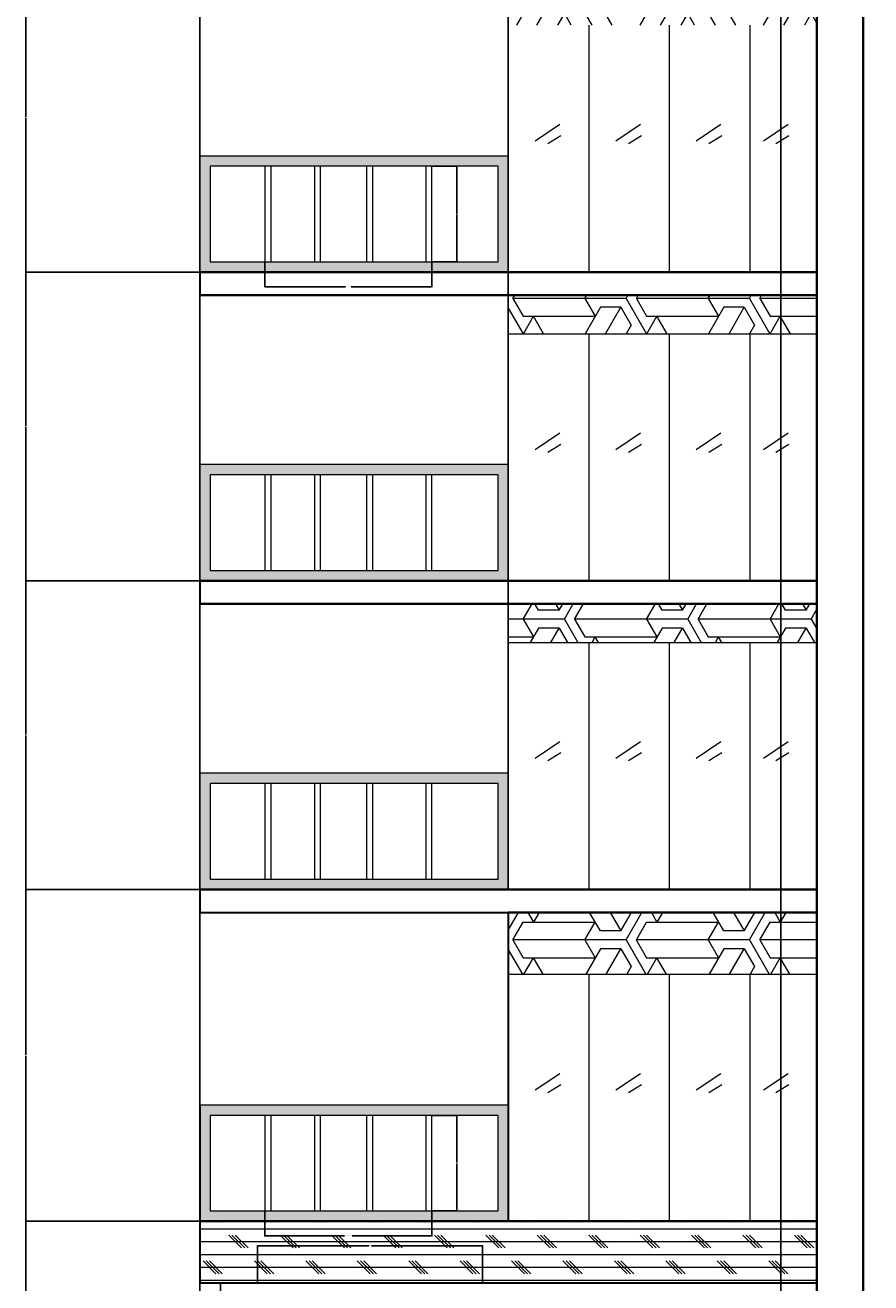
# Model space of a CAD drawing. Units: inches. Extents: x -38 to 698, y -57 to 1364.
# Tile 2 of 5: x -38 to 291, y 227 to 716. Entities that reach past the tile are written whole.
import ezdxf

# ---------------------------------------------------------------- set-up
doc = ezdxf.new("R2010")
doc.units = ezdxf.units.IN
doc.header["$MEASUREMENT"] = 0
for name, color, linetype, lineweight in [('A-ANNO-DIMS', 2, 'Continuous', 18), ('A-ELEV-PATT', 8, 'Continuous', 13), ('A-FLOR', 7, 'Continuous', 30), ('A-FLOR-HRAL', 7, 'Continuous', 20), ('A-GLAZ', 4, 'Continuous', 18), ('A-WALL', 7, 'Continuous', 35), ('A-WALL-PATT', 8, 'Continuous', 13)]:
    doc.layers.add(name, color=color, linetype=linetype, lineweight=lineweight)
doc.styles.get("Standard").update_dxf_attribs({"font": 'arial.ttf'})
doc.dimstyles.get("Standard").update_dxf_attribs({"dimtxt": 0.18, "dimasz": 0.18, "dimexe": 0.18, "dimexo": 0.0625, "dimgap": 0.09, "dimtad": 0, "dimtih": 1, "dimtoh": 1, "dimdec": 4, "dimzin": 0, "dimdsep": 46, "dimtxsty": 'Standard', "dimcen": 0.09, "dimadec": 0, "dimazin": 0, "dimtfac": 1, "dimtdec": 4, "dimtofl": 0, "dimtmove": 0, "dimatfit": 3, "dimfxl": 1, "dimtolj": 1, "dimtzin": 0, "dimarcsym": 0})

# ---------------------------------------------------------------- blocks, each defined once
blk = doc.blocks.new('WINDOW-4L-LH')
for p, q in [((20.81, 96), (20.81, 0)), ((52.11, 96), (52.11, 0)), ((83.42, 96), (83.42, 0)), ((0, 50.99), (9.6, 57.46)), ((31.3, 50.99), (40.9, 57.46)), ((62.61, 50.99), (72.2, 57.46)), ((88.7, 50.99), (98.29, 57.46)), ((4.92, 50.03), (9.96, 53.14)), ((36.22, 50.03), (41.26, 53.14)), ((67.52, 50.03), (72.56, 53.14)), ((93.61, 50.03), (98.65, 53.14))]:
    blk.add_line(p, q)
blk = doc.blocks.new('BALCONY-GUARD-PICKETS')
for p, q in [((0, 37.13), (0, 0)), ((2.41, 0), (2.41, 37.13)), ((19.25, 37.13), (19.25, 0)), ((21.65, 0), (21.65, 37.13)), ((39.53, 37.13), (39.53, 0)), ((41.93, 0), (41.93, 37.13)), ((62.55, 37.13), (62.55, 0)), ((64.96, 0), (64.96, 37.13))]:
    blk.add_line(p, q)
blk = doc.blocks.new('BALCONY-GUARD-PICKETS-BASE')
for p, q in [((19.25, 37.13), (19.25, 0)), ((21.65, 0), (21.65, 37.13)), ((39.53, 37.13), (39.53, 0)), ((41.93, 0), (41.93, 37.13)), ((62.55, 37.13), (62.55, 0)), ((64.96, 0), (64.96, 37.13))]:
    blk.add_line(p, q)
blk.add_lwpolyline([(0, 37.13), (0, 0), (2.41, 0), (2.41, 37.13)])
blk = doc.blocks.new('*D8')
at = {"layer": 'A-ANNO-DIMS', "color": 0, "lineweight": -2, "transparency": 16777216}
for p, q in [((55.02, 624.15), (55.02, 614.29)), ((119.98, 624.15), (119.98, 614.29)), ((55.2, 614.47), (86.4, 614.47)), ((119.8, 614.47), (88.6, 614.47))]:
    blk.add_line(p, q, dxfattribs=at)
at = {"layer": 'A-ANNO-DIMS', "color": 0, "transparency": 16777216}
for points in [[(55.2, 614.5), (55.2, 614.44), (55.02, 614.47)], [(119.8, 614.5), (119.8, 614.44), (119.98, 614.47)]]:
    blk.add_solid(points, dxfattribs=at)
at = {"layer": 'Defpoints', "color": 0, "transparency": 16777216}
for p in [(55.02, 624.21), (119.98, 624.21), (119.98, 614.47)]:
    blk.add_point(p, dxfattribs=at)
at = {"layer": 'A-ANNO-DIMS', "color": 0, "transparency": 16777216, "insert": (87.5, 614.47), "char_height": 0.18, "attachment_point": 5}
blk.add_mtext('\\A1;PICKETS 65 TYP.', dxfattribs=at)
blk = doc.blocks.new('*D9')
at = {"layer": 'A-ANNO-DIMS', "color": 0, "lineweight": -2, "transparency": 16777216}
for p, q in [((120.04, 661.34), (129.91, 661.34)), ((129.73, 661.16), (129.73, 642.96)), ((129.73, 624.39), (129.73, 642.6)), ((120.04, 624.21), (129.91, 624.21))]:
    blk.add_line(p, q, dxfattribs=at)
at = {"layer": 'A-ANNO-DIMS', "color": 0, "transparency": 16777216}
for points in [[(129.7, 661.16), (129.76, 661.16), (129.73, 661.34)], [(129.7, 624.39), (129.76, 624.39), (129.73, 624.21)]]:
    blk.add_solid(points, dxfattribs=at)
at = {"layer": 'Defpoints', "color": 0, "transparency": 16777216}
for p in [(119.98, 661.34), (129.73, 661.34), (119.98, 624.21)]:
    blk.add_point(p, dxfattribs=at)
at = {"layer": 'A-ANNO-DIMS', "color": 0, "transparency": 16777216, "insert": (129.73, 642.78), "char_height": 0.18, "attachment_point": 5}
blk.add_mtext('\\A1;37 TYP.', dxfattribs=at)
blk = doc.blocks.new('*D16')
at = {"layer": 'A-ANNO-DIMS', "color": 0, "lineweight": -2, "transparency": 16777216}
for p, q in [((55.02, 255.15), (55.02, 245.29)), ((119.98, 255.15), (119.98, 245.29)), ((55.2, 245.47), (86.03, 245.47)), ((119.8, 245.47), (88.97, 245.47))]:
    blk.add_line(p, q, dxfattribs=at)
at = {"layer": 'A-ANNO-DIMS', "color": 0, "transparency": 16777216}
for points in [[(55.2, 245.5), (55.2, 245.44), (55.02, 245.47)], [(119.8, 245.5), (119.8, 245.44), (119.98, 245.47)]]:
    blk.add_solid(points, dxfattribs=at)
at = {"layer": 'Defpoints', "color": 0, "transparency": 16777216}
for p in [(55.02, 255.21), (119.98, 255.21), (119.98, 245.47)]:
    blk.add_point(p, dxfattribs=at)
at = {"layer": 'A-ANNO-DIMS', "color": 0, "transparency": 16777216, "insert": (87.5, 245.47), "char_height": 0.18, "attachment_point": 5}
blk.add_mtext('\\A1;BASE PICKETS 65 TYP.', dxfattribs=at)
blk = doc.blocks.new('*D17')
at = {"layer": 'A-ANNO-DIMS', "color": 0, "lineweight": -2, "transparency": 16777216}
for p, q in [((120.04, 292.34), (129.91, 292.34)), ((129.73, 292.16), (129.73, 273.96)), ((129.73, 255.39), (129.73, 273.6)), ((120.04, 255.21), (129.91, 255.21))]:
    blk.add_line(p, q, dxfattribs=at)
at = {"layer": 'A-ANNO-DIMS', "color": 0, "transparency": 16777216}
for points in [[(129.7, 292.16), (129.76, 292.16), (129.73, 292.34)], [(129.7, 255.39), (129.76, 255.39), (129.73, 255.21)]]:
    blk.add_solid(points, dxfattribs=at)
at = {"layer": 'Defpoints', "color": 0, "transparency": 16777216}
for p in [(119.98, 292.34), (129.73, 292.34), (119.98, 255.21)]:
    blk.add_point(p, dxfattribs=at)
at = {"layer": 'A-ANNO-DIMS', "color": 0, "transparency": 16777216, "insert": (129.73, 273.78), "char_height": 0.18, "attachment_point": 5}
blk.add_mtext('\\A1;37 TYP.', dxfattribs=at)
blk = doc.blocks.new('*D20')
at = {"layer": 'A-ANNO-DIMS', "color": 0, "lineweight": -2, "transparency": 16777216}
for p, q in [((52.08, 227.21), (37.56, 227.21)), ((37.74, 227.03), (37.74, 179.4)), ((37.74, 131.39), (37.74, 179.03)), ((52.08, 131.21), (37.56, 131.21))]:
    blk.add_line(p, q, dxfattribs=at)
at = {"layer": 'A-ANNO-DIMS', "color": 0, "transparency": 16777216}
for points in [[(37.71, 227.03), (37.77, 227.03), (37.74, 227.21)], [(37.71, 131.39), (37.77, 131.39), (37.74, 131.21)]]:
    blk.add_solid(points, dxfattribs=at)
at = {"layer": 'Defpoints', "color": 0, "transparency": 16777216}
for p in [(37.74, 227.21), (52.14, 227.21), (52.14, 131.21)]:
    blk.add_point(p, dxfattribs=at)
at = {"layer": 'A-ANNO-DIMS', "color": 0, "transparency": 16777216, "insert": (37.74, 179.21), "char_height": 0.18, "attachment_point": 5}
blk.add_mtext('\\A1;HIGH SCREEN 96 TYP.', dxfattribs=at)
blk = doc.blocks.new('*D21')
at = {"layer": 'A-ANNO-DIMS', "color": 0, "lineweight": -2, "transparency": 16777216}
for p, q in [((52.14, 227.28), (52.14, 241.79)), ((52.32, 241.61), (95.39, 241.61)), ((139.52, 241.61), (96.45, 241.61)), ((139.7, 227.28), (139.7, 241.79))]:
    blk.add_line(p, q, dxfattribs=at)
at = {"layer": 'A-ANNO-DIMS', "color": 0, "transparency": 16777216}
for points in [[(52.32, 241.64), (52.32, 241.58), (52.14, 241.61)], [(139.52, 241.64), (139.52, 241.58), (139.7, 241.61)]]:
    blk.add_solid(points, dxfattribs=at)
at = {"layer": 'Defpoints', "color": 0, "transparency": 16777216}
for p in [(139.7, 241.61), (52.14, 227.21), (139.7, 227.21)]:
    blk.add_point(p, dxfattribs=at)
at = {"layer": 'A-ANNO-DIMS', "color": 0, "transparency": 16777216, "insert": (95.92, 241.61), "char_height": 0.18, "attachment_point": 5}
blk.add_mtext('\\A1;88 TYP.', dxfattribs=at)
blk = doc.blocks.new('*D22')
at = {"layer": 'A-ANNO-DIMS', "color": 0, "lineweight": -2, "transparency": 16777216}
for p, q in [((29.69, 500.15), (29.69, -56.67)), ((629.69, 500.15), (629.69, -56.67)), ((29.87, -56.49), (329.4, -56.49)), ((629.51, -56.49), (329.97, -56.49))]:
    blk.add_line(p, q, dxfattribs=at)
at = {"layer": 'A-ANNO-DIMS', "color": 0, "transparency": 16777216}
for points in [[(29.87, -56.46), (29.87, -56.52), (29.69, -56.49)], [(629.51, -56.46), (629.51, -56.52), (629.69, -56.49)]]:
    blk.add_solid(points, dxfattribs=at)
at = {"layer": 'Defpoints', "color": 0, "transparency": 16777216}
for p in [(29.69, 500.21), (629.69, 500.21), (629.69, -56.49)]:
    blk.add_point(p, dxfattribs=at)
at = {"layer": 'A-ANNO-DIMS', "color": 0, "transparency": 16777216, "insert": (329.69, -56.49), "char_height": 0.18, "attachment_point": 5}
blk.add_mtext('\\A1;600', dxfattribs=at)
blk = doc.blocks.new('*D24')
at = {"layer": 'A-ANNO-DIMS', "color": 0, "lineweight": -2, "transparency": 16777216}
for p, q in [((29.69, 1100.15), (29.69, -56.67)), ((269.69, 1100.15), (269.69, -56.67)), ((29.87, -56.49), (149.4, -56.49)), ((269.51, -56.49), (149.98, -56.49))]:
    blk.add_line(p, q, dxfattribs=at)
at = {"layer": 'A-ANNO-DIMS', "color": 0, "transparency": 16777216}
for points in [[(29.87, -56.46), (29.87, -56.52), (29.69, -56.49)], [(269.51, -56.46), (269.51, -56.52), (269.69, -56.49)]]:
    blk.add_solid(points, dxfattribs=at)
at = {"layer": 'Defpoints', "color": 0, "transparency": 16777216}
for p in [(29.69, 1100.21), (269.69, 1100.21), (269.69, -56.49)]:
    blk.add_point(p, dxfattribs=at)
at = {"layer": 'A-ANNO-DIMS', "color": 0, "transparency": 16777216, "insert": (149.69, -56.49), "char_height": 0.18, "attachment_point": 5}
blk.add_mtext('\\A1;240', dxfattribs=at)
blk = doc.blocks.new('*D25')
at = {"layer": 'A-ANNO-DIMS', "color": 0, "lineweight": -2, "transparency": 16777216}
for p, q in [((269.69, 1100.15), (269.69, -56.67)), ((389.69, 1100.15), (389.69, -56.67)), ((269.87, -56.49), (329.41, -56.49)), ((389.51, -56.49), (329.97, -56.49))]:
    blk.add_line(p, q, dxfattribs=at)
at = {"layer": 'A-ANNO-DIMS', "color": 0, "transparency": 16777216}
for points in [[(269.87, -56.46), (269.87, -56.52), (269.69, -56.49)], [(389.51, -56.46), (389.51, -56.52), (389.69, -56.49)]]:
    blk.add_solid(points, dxfattribs=at)
at = {"layer": 'Defpoints', "color": 0, "transparency": 16777216}
for p in [(269.69, 1100.21), (389.69, 1100.21), (389.69, -56.49)]:
    blk.add_point(p, dxfattribs=at)
at = {"layer": 'A-ANNO-DIMS', "color": 0, "transparency": 16777216, "insert": (329.69, -56.49), "char_height": 0.18, "attachment_point": 5}
blk.add_mtext('\\A1;120', dxfattribs=at)
blk = doc.blocks.new('*D27')
at = {"layer": 'A-ANNO-DIMS', "color": 0, "lineweight": -2, "transparency": 16777216}
for p, q in [((149.69, 380.28), (149.69, 1362.92)), ((149.87, 1362.74), (209.41, 1362.74)), ((269.51, 1362.74), (209.97, 1362.74)), ((269.69, 380.28), (269.69, 1362.92))]:
    blk.add_line(p, q, dxfattribs=at)
at = {"layer": 'A-ANNO-DIMS', "color": 0, "transparency": 16777216}
for points in [[(149.87, 1362.77), (149.87, 1362.71), (149.69, 1362.74)], [(269.51, 1362.77), (269.51, 1362.71), (269.69, 1362.74)]]:
    blk.add_solid(points, dxfattribs=at)
at = {"layer": 'Defpoints', "color": 0, "transparency": 16777216}
for p in [(269.69, 1362.74), (149.69, 380.21), (269.69, 380.21)]:
    blk.add_point(p, dxfattribs=at)
at = {"layer": 'A-ANNO-DIMS', "color": 0, "transparency": 16777216, "insert": (209.69, 1362.74), "char_height": 0.18, "attachment_point": 5}
blk.add_mtext('\\A1;120', dxfattribs=at)
blk = doc.blocks.new('*D30')
at = {"layer": 'A-ANNO-DIMS', "color": 0, "lineweight": -2, "transparency": 16777216}
for p, q in [((29.62, 251.21), (-38.19, 251.21)), ((-38.01, 251.03), (-38.01, 191.4)), ((-38.01, 131.39), (-38.01, 191.03)), ((29.62, 131.21), (-38.19, 131.21))]:
    blk.add_line(p, q, dxfattribs=at)
at = {"layer": 'A-ANNO-DIMS', "color": 0, "transparency": 16777216}
for points in [[(-38.04, 251.03), (-37.98, 251.03), (-38.01, 251.21)], [(-38.04, 131.39), (-37.98, 131.39), (-38.01, 131.21)]]:
    blk.add_solid(points, dxfattribs=at)
at = {"layer": 'Defpoints', "color": 0, "transparency": 16777216}
for p in [(-38.01, 251.21), (29.69, 251.21), (29.69, 131.21)]:
    blk.add_point(p, dxfattribs=at)
at = {"layer": 'A-ANNO-DIMS', "color": 0, "transparency": 16777216, "insert": (-38.01, 191.21), "char_height": 0.18, "attachment_point": 5}
blk.add_mtext('\\A1;120', dxfattribs=at)
blk = doc.blocks.new('*D31')
at = {"layer": 'A-ANNO-DIMS', "color": 0, "lineweight": -2, "transparency": 16777216}
for p, q in [((29.62, 380.21), (-38.19, 380.21)), ((-38.01, 380.03), (-38.01, 315.9)), ((-38.01, 251.39), (-38.01, 315.53)), ((29.62, 251.21), (-38.19, 251.21))]:
    blk.add_line(p, q, dxfattribs=at)
at = {"layer": 'A-ANNO-DIMS', "color": 0, "transparency": 16777216}
for points in [[(-38.04, 380.03), (-37.98, 380.03), (-38.01, 380.21)], [(-38.04, 251.39), (-37.98, 251.39), (-38.01, 251.21)]]:
    blk.add_solid(points, dxfattribs=at)
at = {"layer": 'Defpoints', "color": 0, "transparency": 16777216}
for p in [(-38.01, 380.21), (29.69, 380.21), (29.69, 251.21)]:
    blk.add_point(p, dxfattribs=at)
at = {"layer": 'A-ANNO-DIMS', "color": 0, "transparency": 16777216, "insert": (-38.01, 315.71), "char_height": 0.18, "attachment_point": 5}
blk.add_mtext('\\A1;129', dxfattribs=at)
blk = doc.blocks.new('*D32')
at = {"layer": 'A-ANNO-DIMS', "color": 0, "lineweight": -2, "transparency": 16777216}
for p, q in [((29.62, 500.21), (-38.19, 500.21)), ((-38.01, 500.03), (-38.01, 440.4)), ((-38.01, 380.39), (-38.01, 440.03)), ((29.62, 380.21), (-38.19, 380.21))]:
    blk.add_line(p, q, dxfattribs=at)
at = {"layer": 'A-ANNO-DIMS', "color": 0, "transparency": 16777216}
for points in [[(-38.04, 500.03), (-37.98, 500.03), (-38.01, 500.21)], [(-38.04, 380.39), (-37.98, 380.39), (-38.01, 380.21)]]:
    blk.add_solid(points, dxfattribs=at)
at = {"layer": 'Defpoints', "color": 0, "transparency": 16777216}
for p in [(-38.01, 500.21), (29.69, 500.21), (29.69, 380.21)]:
    blk.add_point(p, dxfattribs=at)
at = {"layer": 'A-ANNO-DIMS', "color": 0, "transparency": 16777216, "insert": (-38.01, 440.21), "char_height": 0.18, "attachment_point": 5}
blk.add_mtext('\\A1;120', dxfattribs=at)
blk = doc.blocks.new('*D33')
at = {"layer": 'A-ANNO-DIMS', "color": 0, "lineweight": -2, "transparency": 16777216}
for p, q in [((29.62, 620.21), (-38.19, 620.21)), ((-38.01, 620.03), (-38.01, 560.4)), ((-38.01, 500.39), (-38.01, 560.03)), ((29.62, 500.21), (-38.19, 500.21))]:
    blk.add_line(p, q, dxfattribs=at)
at = {"layer": 'A-ANNO-DIMS', "color": 0, "transparency": 16777216}
for points in [[(-38.04, 620.03), (-37.98, 620.03), (-38.01, 620.21)], [(-38.04, 500.39), (-37.98, 500.39), (-38.01, 500.21)]]:
    blk.add_solid(points, dxfattribs=at)
at = {"layer": 'Defpoints', "color": 0, "transparency": 16777216}
for p in [(-38.01, 620.21), (29.69, 620.21), (29.69, 500.21)]:
    blk.add_point(p, dxfattribs=at)
at = {"layer": 'A-ANNO-DIMS', "color": 0, "transparency": 16777216, "insert": (-38.01, 560.21), "char_height": 0.18, "attachment_point": 5}
blk.add_mtext('\\A1;120', dxfattribs=at)
blk = doc.blocks.new('*D34')
at = {"layer": 'A-ANNO-DIMS', "color": 0, "lineweight": -2, "transparency": 16777216}
for p, q in [((29.62, 740.21), (-38.19, 740.21)), ((-38.01, 740.03), (-38.01, 680.4)), ((-38.01, 620.39), (-38.01, 680.03)), ((29.62, 620.21), (-38.19, 620.21))]:
    blk.add_line(p, q, dxfattribs=at)
at = {"layer": 'A-ANNO-DIMS', "color": 0, "transparency": 16777216}
for points in [[(-38.04, 740.03), (-37.98, 740.03), (-38.01, 740.21)], [(-38.04, 620.39), (-37.98, 620.39), (-38.01, 620.21)]]:
    blk.add_solid(points, dxfattribs=at)
at = {"layer": 'Defpoints', "color": 0, "transparency": 16777216}
for p in [(-38.01, 740.21), (29.69, 740.21), (29.69, 620.21)]:
    blk.add_point(p, dxfattribs=at)
at = {"layer": 'A-ANNO-DIMS', "color": 0, "transparency": 16777216, "insert": (-38.01, 680.21), "char_height": 0.18, "attachment_point": 5}
blk.add_mtext('\\A1;120', dxfattribs=at)
blk = doc.blocks.new('*D48')
at = {"layer": 'A-ANNO-DIMS', "color": 0, "lineweight": -2, "transparency": 16777216}
for p, q in [((255.72, 101.28), (255.72, 1362.92)), ((255.9, 1362.74), (328.99, 1362.74)), ((402.85, 1362.74), (329.76, 1362.74)), ((403.03, 101.28), (403.03, 1362.92))]:
    blk.add_line(p, q, dxfattribs=at)
at = {"layer": 'A-ANNO-DIMS', "color": 0, "transparency": 16777216}
for points in [[(255.9, 1362.77), (255.9, 1362.71), (255.72, 1362.74)], [(402.85, 1362.77), (402.85, 1362.71), (403.03, 1362.74)]]:
    blk.add_solid(points, dxfattribs=at)
at = {"layer": 'Defpoints', "color": 0, "transparency": 16777216}
for p in [(403.03, 1362.74), (255.72, 101.21), (403.03, 101.21)]:
    blk.add_point(p, dxfattribs=at)
at = {"layer": 'A-ANNO-DIMS', "color": 0, "transparency": 16777216, "insert": (329.37, 1362.74), "char_height": 0.18, "attachment_point": 5}
blk.add_mtext('\\A1;147.3', dxfattribs=at)
blk = doc.blocks.new('*D52')
at = {"layer": 'A-ANNO-DIMS', "color": 0, "lineweight": -2, "transparency": 16777216}
for p, q in [((287.69, 1294.97), (287.69, -56.67)), ((269.69, 1282.97), (269.69, -56.67)), ((269.87, -56.49), (278.47, -56.49)), ((287.51, -56.49), (278.9, -56.49))]:
    blk.add_line(p, q, dxfattribs=at)
at = {"layer": 'A-ANNO-DIMS', "color": 0, "transparency": 16777216}
for points in [[(269.87, -56.46), (269.87, -56.52), (269.69, -56.49)], [(287.51, -56.46), (287.51, -56.52), (287.69, -56.49)]]:
    blk.add_solid(points, dxfattribs=at)
at = {"layer": 'Defpoints', "color": 0, "transparency": 16777216}
for p in [(287.69, 1295.04), (269.69, 1283.04), (287.69, -56.49)]:
    blk.add_point(p, dxfattribs=at)
at = {"layer": 'A-ANNO-DIMS', "color": 0, "transparency": 16777216, "insert": (278.69, -56.49), "char_height": 0.18, "attachment_point": 5}
blk.add_mtext('\\A1;18', dxfattribs=at)

msp = doc.modelspace()

# ---------------------------------------------------------------- hatches: boundary and pattern name
at = {"layer": 'A-ELEV-PATT', "transparency": 33554562}
h = msp.add_hatch(dxfattribs=at)
h.set_pattern_fill('HONEY', color=256, scale=40)
h.set_pattern_definition([(0, (-116.5534, -96.733), (7.5, 4.330127), [5, -10]), (120, (-116.5534, -96.733), (-7.5, 4.330127), [5, -10]), (60, (-116.5534, -96.733), (2e-15, 8.660254), [-10, 5])])
h.paths.add_polyline_path([(629.0638, 1145.3406), (509.0638, 1145.3406), (509.0638, 1100.2149), (629.0638, 1100.2149)])
h.paths.add_polyline_path([(625.0638, 1141.3406), (625.0638, 1104.2149), (513.0638, 1104.2149), (513.0638, 1141.3406)], flags=16)
h.paths.add_polyline_path([(629.0638, 1025.3406), (509.0638, 1025.3406), (509.0638, 980.2149), (629.0638, 980.2149)])
h.paths.add_polyline_path([(625.0638, 1021.3406), (625.0638, 984.2149), (513.0638, 984.2149), (513.0638, 1021.3406)], flags=16)
h.paths.add_polyline_path([(629.0638, 905.3406), (509.0638, 905.3406), (509.0638, 860.2149), (629.0638, 860.2149)])
h.paths.add_polyline_path([(625.0638, 901.3406), (625.0638, 864.2149), (513.0638, 864.2149), (513.0638, 901.3406)], flags=16)
h.paths.add_polyline_path([(629.0638, 785.3406), (509.0638, 785.3406), (509.0638, 740.2149), (629.0638, 740.2149)])
h.paths.add_polyline_path([(625.0638, 781.3406), (625.0638, 744.2149), (513.0638, 744.2149), (513.0638, 781.3406)], flags=16)
h.paths.add_polyline_path([(629.0638, 665.3406), (509.0638, 665.3406), (509.0638, 620.2149), (629.0638, 620.2149)])
h.paths.add_polyline_path([(625.0638, 661.3406), (625.0638, 624.2149), (513.0638, 624.2149), (513.0638, 661.3406)], flags=16)
h.paths.add_polyline_path([(629.0638, 545.3406), (509.0638, 545.3406), (509.0638, 500.2149), (629.0638, 500.2149)])
h.paths.add_polyline_path([(625.0638, 541.3406), (625.0638, 504.2149), (513.0638, 504.2149), (513.0638, 541.3406)], flags=16)
h.paths.add_polyline_path([(629.0638, 425.3406), (509.0638, 425.3406), (509.0638, 380.2149), (629.0638, 380.2149)])
h.paths.add_polyline_path([(625.0638, 421.3406), (625.0638, 384.2149), (513.0638, 384.2149), (513.0638, 421.3406)], flags=16)
h.paths.add_polyline_path([(629.0638, 296.3406), (509.0638, 296.3406), (509.0638, 251.2149), (629.0638, 251.2149)])
h.paths.add_polyline_path([(625.0638, 292.3406), (625.0638, 255.2149), (513.0638, 255.2149), (513.0638, 292.3406)], flags=16)
h.paths.add_polyline_path([(149.6854, 296.3406), (29.6854, 296.3406), (29.6854, 251.2149), (149.6854, 251.2149)])
h.paths.add_polyline_path([(145.6854, 292.3406), (145.6854, 255.2149), (33.6854, 255.2149), (33.6854, 292.3406)], flags=16)
h.paths.add_polyline_path([(149.6854, 425.3406), (29.6854, 425.3406), (29.6854, 380.2149), (149.6854, 380.2149)])
h.paths.add_polyline_path([(145.6854, 421.3406), (145.6854, 384.2149), (33.6854, 384.2149), (33.6854, 421.3406)], flags=16)
h.paths.add_polyline_path([(149.6854, 545.3406), (29.6854, 545.3406), (29.6854, 500.2149), (149.6854, 500.2149)])
h.paths.add_polyline_path([(33.6854, 504.2149), (33.6854, 541.3406), (145.6854, 541.3406), (145.6854, 504.2149)], flags=16)
h.paths.add_polyline_path([(149.6854, 665.3406), (29.6854, 665.3406), (29.6854, 620.2149), (149.6854, 620.2149)])
h.paths.add_polyline_path([(33.6854, 624.2149), (33.6854, 661.3406), (145.6854, 661.3406), (145.6854, 624.2149)], flags=16)
h.paths.add_polyline_path([(149.6854, 785.3406), (29.6854, 785.3406), (29.6854, 740.2149), (149.6854, 740.2149)])
h.paths.add_polyline_path([(33.6854, 744.2149), (33.6854, 781.3406), (145.6854, 781.3406), (145.6854, 744.2149)], flags=16)
h.paths.add_polyline_path([(149.6854, 905.3406), (29.6854, 905.3406), (29.6854, 860.2149), (149.6854, 860.2149)])
h.paths.add_polyline_path([(145.6854, 901.3406), (145.6854, 864.2149), (33.6854, 864.2149), (33.6854, 901.3406)], flags=16)
h.paths.add_polyline_path([(149.6854, 1025.3406), (29.6854, 1025.3406), (29.6854, 980.2149), (149.6854, 980.2149)])
h.paths.add_polyline_path([(33.6854, 984.2149), (33.6854, 1021.3406), (145.6854, 1021.3406), (145.6854, 984.2149)], flags=16)
h.paths.add_polyline_path([(149.6854, 1145.3406), (29.6854, 1145.3406), (29.6854, 1100.2149), (149.6854, 1100.2149)])
h.paths.add_polyline_path([(33.6854, 1104.2149), (33.6854, 1141.3406), (145.6854, 1141.3406), (145.6854, 1104.2149)], flags=16)
h = msp.add_hatch(dxfattribs=at)
h.set_pattern_fill('CORK', color=256, scale=40)
h.set_pattern_definition([(0, (-116.5534, -96.733), (0, 5), []), (135, (-114.053, -99.233), (-10, -10), [7.07107, -7.07107]), (135, (-112.803, -99.233), (-10, -10), [7.07107, -7.07107]), (135, (-111.553, -99.233), (-10, -10), [7.07107, -7.07107])])
h.paths.add_polyline_path([(269.6854, 131.2149), (29.6854, 131.2149), (29.6854, 107.2149), (269.6854, 107.2149)])
h.paths.add_polyline_path([(269.6854, 251.2149), (29.6854, 251.2149), (29.6854, 227.2149), (269.6854, 227.2149)])
h.paths.add_polyline_path([(629.6854, 251.2149), (389.6854, 251.2149), (389.6854, 227.2149), (629.6854, 227.2149)])
h.paths.add_polyline_path([(629.6854, 131.2149), (389.6854, 131.2149), (389.6854, 107.2149), (409.029, 107.2149), (629.6854, 107.2149)])
at = {"layer": 'A-WALL-PATT', "transparency": 33554562}
h = msp.add_hatch(dxfattribs=at)
h.set_pattern_fill('ESCHER', color=256, scale=40)
h.set_pattern_definition([(60, (-116.553, -96.733), (-48, -1e-08), [44, -4]), (180, (-116.553, -96.733), (24, -41.5692), [44, -4]), (300, (-116.553, -96.733), (48, -1e-08), [44, -4]), (60, (-112.553, -96.733), (-48, -1e-08), [8, -40]), (300, (-112.553, -96.733), (48, -1e-08), [8, -40]), (60, (-118.553, -93.27), (-48, -1e-08), [8, -40]), (180, (-118.553, -93.27), (24, -41.5692), [8, -40]), (300, (-118.553, -100.197), (48, -1e-08), [8, -40]), (180, (-118.553, -100.197), (24, -41.5692), [8, -40]), (60, (-132.553, -96.733), (-48, -1e-08), [8, -40]), (300, (-132.553, -96.733), (48, -1e-08), [8, -40]), (60, (-108.553, -110.59), (-48, -1e-08), [8, -40]), (180, (-108.553, -110.59), (24, -41.5692), [8, -40]), (300, (-108.553, -82.877), (48, -1e-08), [8, -40]), (180, (-108.553, -82.877), (24, -41.5692), [8, -40]), (0, (-108.553, -89.805), (-24, 41.5692), [28, -20]), (0, (-108.553, -103.66), (-24, 41.5692), [28, -20]), (120, (-114.553, -86.34), (-48, 1e-08), [28, -20]), (120, (-126.553, -93.27), (-48, 1e-08), [28, -20]), (240, (-126.553, -100.197), (24, -41.5692), [28, -20]), (240, (-114.553, -107.125), (24, -41.5692), [28, -20])])
h.paths.add_polyline_path([(269.6854, 371.2149), (149.6854, 371.2149), (149.6854, 347.2149), (269.6854, 347.2149)])
h.paths.add_polyline_path([(509.0638, 371.2149), (389.6854, 371.2149), (389.6854, 347.2149), (509.0638, 347.2149)])
h.paths.add_polyline_path([(269.6854, 491.2149), (149.6854, 491.2149), (149.6854, 476.2149), (269.6854, 476.2149)])
h.paths.add_polyline_path([(509.0638, 491.2149), (389.6854, 491.2149), (389.6854, 476.2149), (509.0638, 476.2149)])
h.paths.add_polyline_path([(509.0638, 611.2149), (389.6854, 611.2149), (389.6854, 596.2149), (509.0638, 596.2149)])
h.paths.add_polyline_path([(269.6854, 611.2149), (149.6854, 611.2149), (149.6854, 596.2149), (269.6854, 596.2149)])
h.paths.add_polyline_path([(269.6854, 731.2149), (149.6854, 731.2149), (149.6854, 716.2149), (269.6854, 716.2149)])
h.paths.add_polyline_path([(509.0638, 731.2149), (389.6854, 731.2149), (389.6854, 716.2149), (509.0638, 716.2149)])
h.paths.add_polyline_path([(509.0638, 851.2149), (389.6854, 851.2149), (389.6854, 836.2149), (509.0638, 836.2149)])
h.paths.add_polyline_path([(269.6854, 851.2149), (149.6854, 851.2149), (149.6854, 836.2149), (269.6854, 836.2149)])
h.paths.add_polyline_path([(269.6854, 971.2149), (149.6854, 971.2149), (149.6854, 956.2149), (269.6854, 956.2149)])
h.paths.add_polyline_path([(509.0638, 971.2149), (389.6854, 971.2149), (389.6854, 956.2149), (509.0638, 956.2149)])
h.paths.add_polyline_path([(509.0638, 1091.2149), (389.6854, 1091.2149), (389.6854, 1076.2149), (509.0638, 1076.2149)])
h.paths.add_polyline_path([(269.6854, 1091.2149), (149.6854, 1091.2149), (149.6854, 1076.2149), (269.6854, 1076.2149)])

# ---------------------------------------------------------------- linework, layer by layer
at = {"layer": 'A-FLOR'}
for points in [[(29.6854, 620.2149), (269.6854, 620.2149), (29.6854, 620.2149), (29.6854, 611.2149), (269.6854, 611.2149), (29.6854, 611.2149)], [(29.6854, 500.2149), (269.6854, 500.2149), (29.6854, 500.2149), (29.6854, 491.2149), (269.6854, 491.2149), (29.6854, 491.2149)], [(29.6854, 380.2149), (269.6854, 380.2149), (29.6854, 380.2149), (29.6854, 371.2149), (149.6854, 371.2149)], [(29.6854, 371.2149), (269.6854, 371.2149), (149.6854, 371.2149), (149.6854, 251.2149)], [(29.6854, 296.3406), (29.6854, 251.2149), (29.6854, 227.2149), (269.6854, 227.2149)]]:
    msp.add_lwpolyline(points, dxfattribs=at)
msp.add_lwpolyline([(29.6854, 251.2149), (269.6854, 251.2149)], close=True, dxfattribs=at)
at = {"layer": 'A-FLOR-HRAL'}
for points in [[(149.6854, 665.3406), (29.6854, 665.3406), (29.6854, 620.2149), (149.6854, 620.2149)], [(145.6854, 661.3406), (33.6854, 661.3406), (33.6854, 624.2149), (145.6854, 624.2149)], [(149.6854, 545.3406), (29.6854, 545.3406), (29.6854, 500.2149), (149.6854, 500.2149)], [(145.6854, 541.3406), (33.6854, 541.3406), (33.6854, 504.2149), (145.6854, 504.2149)], [(149.6854, 425.3406), (29.6854, 425.3406), (29.6854, 380.2149), (149.6854, 380.2149)], [(145.6854, 421.3406), (33.6854, 421.3406), (33.6854, 384.2149), (145.6854, 384.2149)], [(149.6854, 296.3406), (29.6854, 296.3406), (29.6854, 251.2149), (149.6854, 251.2149)], [(145.6854, 292.3406), (33.6854, 292.3406), (33.6854, 255.2149), (145.6854, 255.2149)]]:
    msp.add_lwpolyline(points, close=True, dxfattribs=at)
at = {"layer": 'A-GLAZ'}
for p, q in [((149.6854, 596.2149), (269.6854, 596.2149)), ((149.6854, 476.2149), (269.6854, 476.2149)), ((149.6854, 347.2149), (269.6854, 347.2149))]:
    msp.add_line(p, q, dxfattribs=at)
for points in [[(149.6854, 620.2149), (149.6854, 731.2149)], [(149.6854, 500.2149), (149.6854, 611.2149)], [(149.6854, 380.2149), (149.6854, 491.2149)]]:
    msp.add_lwpolyline(points, close=True, dxfattribs=at)
at = {"layer": 'A-WALL'}
msp.add_lwpolyline([(269.6854, 107.2149), (269.6854, 851.2149), (269.6854, 971.2149), (269.6854, 1283.0353), (141.3895, 1283.0353), (141.3895, 1295.0353), (287.6854, 1295.0353), (287.6854, 971.2149), (287.6854, 851.2149), (287.6854, 107.2149)], dxfattribs=at)

# ---------------------------------------------------------------- block references
at = {"layer": 'A-FLOR-HRAL'}
for name, p in [('BALCONY-GUARD-PICKETS', (55.02, 624.215)), ('BALCONY-GUARD-PICKETS', (55.02, 504.215)), ('BALCONY-GUARD-PICKETS', (55.02, 384.215)), ('BALCONY-GUARD-PICKETS-BASE', (55.02, 255.215))]:
    msp.add_blockref(name, p, dxfattribs=at)
at = {"layer": 'A-GLAZ'}
for p in [(160.18, 620.215), (160.18, 500.215), (160.18, 380.215), (160.18, 251.215)]:
    msp.add_blockref('WINDOW-4L-LH', p, dxfattribs=at)

# ---------------------------------------------------------------- dimensions: what is measured, and where the dimension line sits
at = {"layer": 'A-ANNO-DIMS'}
for base, p1, p2, override, picture, middle in [((269.6854, 1362.7353), (149.6854, 380.2149), (269.6854, 380.2149), {"dimdec": 0, "dimlfac": 1, "dimrnd": 0, "dimzin": 0, "dimdsep": 46, "dimlunit": 2}, '*D27', (209.6854, 1362.7353)), ((403.029, 1362.7353), (255.7202, 101.2149), (403.029, 101.2149), {"dimdec": 1, "dimlfac": 1, "dimrnd": 0, "dimzin": 0, "dimdsep": 46, "dimlunit": 2}, '*D48', (329.3746, 1362.7353)), ((287.6854, -56.4851), (269.6854, 1283.0353), (287.6854, 1295.0353), {"dimdec": 0, "dimlfac": 1, "dimrnd": 0, "dimzin": 0, "dimdsep": 46, "dimlunit": 2}, '*D52', (278.6854, -56.4851)), ((269.6854, -56.4851), (29.6854, 1100.2149), (269.6854, 1100.2149), {"dimdec": 0, "dimlfac": 1, "dimrnd": 0, "dimzin": 0, "dimdsep": 46, "dimlunit": 2}, '*D24', (149.6854, -56.4851)), ((389.6854, -56.4851), (269.6854, 1100.2149), (389.6854, 1100.2149), {"dimdec": 0, "dimlfac": 1, "dimrnd": 0, "dimzin": 0, "dimdsep": 46, "dimlunit": 2}, '*D25', (329.6854, -56.4851)), ((629.6854, -56.4851), (29.6854, 500.2149), (629.6854, 500.2149), {"dimdec": 0, "dimlfac": 1, "dimrnd": 0, "dimzin": 0, "dimdsep": 46, "dimlunit": 2}, '*D22', (329.6854, -56.4851))]:
    dim = msp.add_linear_dim(base=base, p1=p1, p2=p2, dimstyle='Standard', override=override, dxfattribs=at)
    dim.commit()
    dim.dimension.update_dxf_attribs({"geometry": picture, "text_midpoint": middle})
for base, p1, p2, picture, middle in [((-38.0146, 740.2149), (29.6854, 620.2149), (29.6854, 740.2149), '*D34', (-38.0146, 680.2149)), ((-38.0146, 620.2149), (29.6854, 500.2149), (29.6854, 620.2149), '*D33', (-38.0146, 560.2149)), ((-38.0146, 500.2149), (29.6854, 380.2149), (29.6854, 500.2149), '*D32', (-38.0146, 440.2149)), ((-38.0146, 380.2149), (29.6854, 251.2149), (29.6854, 380.2149), '*D31', (-38.0146, 315.7149)), ((-38.0146, 251.2149), (29.6854, 131.2149), (29.6854, 251.2149), '*D30', (-38.0146, 191.2149))]:
    dim = msp.add_linear_dim(base=base, p1=p1, p2=p2, angle=90, dimstyle='Standard', override={"dimdec": 0, "dimlfac": 1, "dimrnd": 0, "dimzin": 0, "dimdsep": 46, "dimlunit": 2}, dxfattribs=at)
    dim.commit()
    dim.dimension.update_dxf_attribs({"geometry": picture, "text_midpoint": middle})
for base, p1, p2, text, picture, middle in [((129.7251, 661.3406), (119.9809, 624.2149), (119.9809, 661.3406), '<> TYP.', '*D9', (129.7251, 642.7777)), ((129.7251, 292.3406), (119.9809, 255.2149), (119.9809, 292.3406), '<> TYP.', '*D17', (129.7251, 273.7777)), ((37.7408, 227.2149), (52.1408, 131.2149), (52.1408, 227.2149), 'HIGH SCREEN <> TYP.', '*D20', (37.7408, 179.2149))]:
    dim = msp.add_linear_dim(base=base, p1=p1, p2=p2, angle=90, text=text, dimstyle='Standard', override={"dimdec": 0, "dimlfac": 1, "dimrnd": 0, "dimzin": 0, "dimdsep": 46, "dimlunit": 2}, dxfattribs=at)
    dim.commit()
    dim.dimension.update_dxf_attribs({"geometry": picture, "text_midpoint": middle})
for base, p1, p2, text, picture, middle in [((119.9809, 614.4707), (55.0198, 624.2149), (119.9809, 624.2149), 'PICKETS <> TYP.', '*D8', (87.5003, 614.4707)), ((119.9809, 245.4707), (55.0198, 255.2149), (119.9809, 255.2149), 'BASE PICKETS <> TYP.', '*D16', (87.5003, 245.4707)), ((139.7028, 241.6149), (52.1408, 227.2149), (139.7028, 227.2149), '<> TYP.', '*D21', (95.9218, 241.6149))]:
    dim = msp.add_linear_dim(base=base, p1=p1, p2=p2, text=text, dimstyle='Standard', override={"dimdec": 0, "dimlfac": 1, "dimrnd": 0, "dimzin": 0, "dimdsep": 46, "dimlunit": 2}, dxfattribs=at)
    dim.commit()
    dim.dimension.update_dxf_attribs({"geometry": picture, "text_midpoint": middle})

doc.saveas('drawing.dxf')
